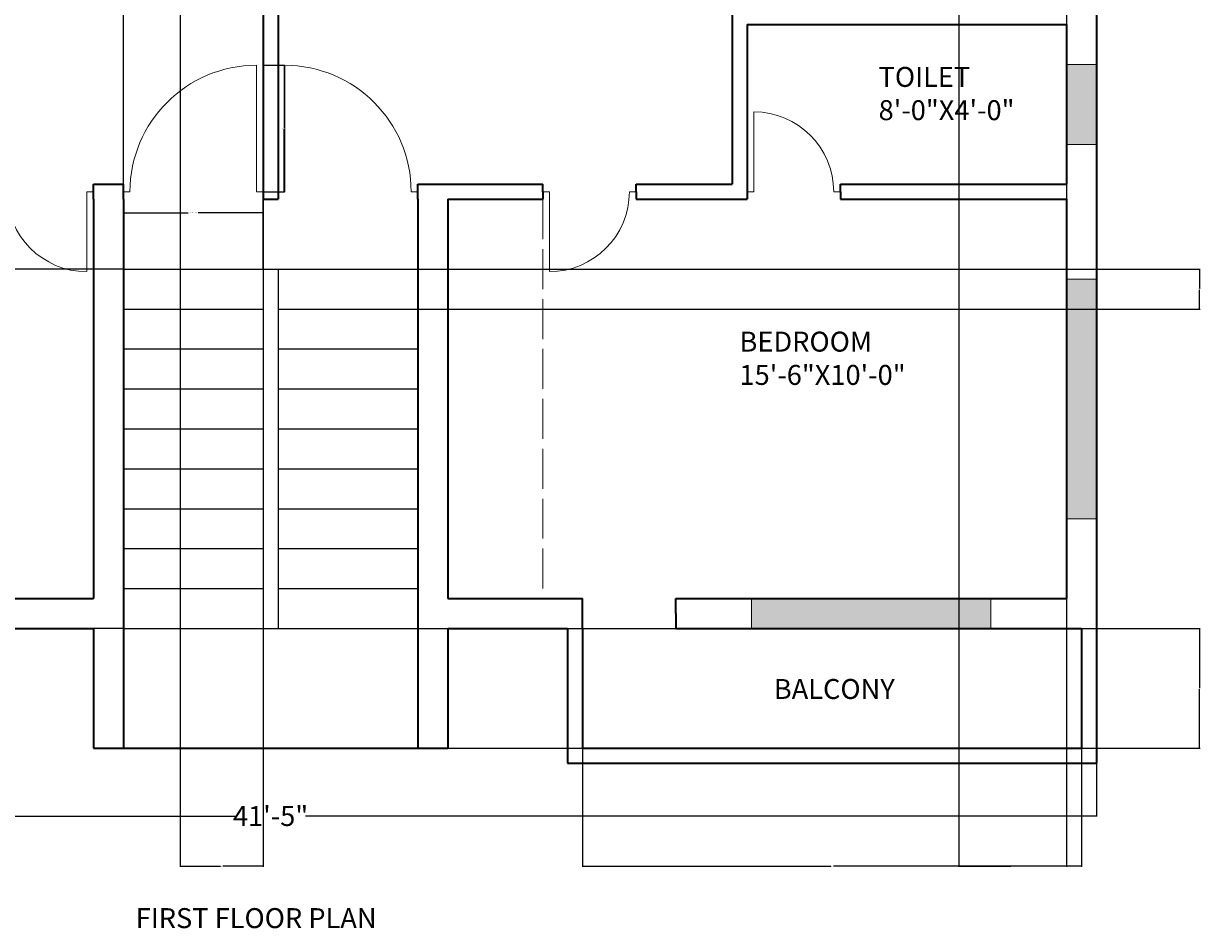
# Model space of a CAD drawing. Units: inches. Extents: x -89 to 565, y -517 to 71.
# Tile 2 of 3: x 211 to 565, y -517 to -245. Entities that reach past the tile are written whole.
import ezdxf

# ---------------------------------------------------------------- set-up
doc = ezdxf.new("R2010")
doc.units = ezdxf.units.IN
doc.header["$MEASUREMENT"] = 0
doc.linetypes.add('ACAD_ISO02W100', pattern=[15, 12, -3])
for name, color, linetype, lineweight in [('A-ANNO-DIMS', 2, 'Continuous', 18), ('A-ANNO-TEXT', 7, 'Continuous', 25), ('A-AREA-IDEN', 7, 'Continuous', 18), ('A-DOOR', 4, 'Continuous', 18), ('A-FLOR-OVHD', 8, 'ACAD_ISO02W100', 18), ('A-FLOR-STRS', 7, 'Continuous', 25), ('A-GLAZ', 3, 'Continuous', 18), ('A-GLAZ-PATT', 9, 'Continuous', 13), ('A-WALL', 7, 'Continuous', 35)]:
    doc.layers.add(name, color=color, linetype=linetype, lineweight=lineweight)
doc.styles.get("Standard").update_dxf_attribs({"font": 'arial.ttf'})
doc.dimstyles.get("Standard").update_dxf_attribs({"dimtxt": 0.18, "dimasz": 0.18, "dimexe": 0.18, "dimexo": 0.0625, "dimgap": 0.09, "dimtad": 0, "dimtih": 1, "dimtoh": 1, "dimdec": 0, "dimzin": 0, "dimdsep": 46, "dimlunit": 3, "dimtxsty": 'Standard', "dimcen": 0.09, "dimadec": 0, "dimazin": 0, "dimtfac": 1, "dimtdec": 0, "dimtofl": 0, "dimtmove": 0, "dimatfit": 3, "dimfxl": 1, "dimtolj": 1, "dimtzin": 0, "dimarcsym": 0})

# ---------------------------------------------------------------- blocks, each defined once
blk = doc.blocks.new('*D2')
at = {"layer": 'A-ANNO-DIMS', "color": 0, "lineweight": -2, "transparency": 16777216}
for p, q in [((37.09, -467.65), (37.09, -483.62)), ((533.59, -467.65), (533.59, -483.62)), ((37.27, -483.44), (274.83, -483.44)), ((533.41, -483.44), (295.86, -483.44))]:
    blk.add_line(p, q, dxfattribs=at)
at = {"layer": 'A-ANNO-DIMS', "color": 0, "transparency": 16777216}
for points in [[(37.27, -483.41), (37.27, -483.47), (37.09, -483.44)], [(533.41, -483.41), (533.41, -483.47), (533.59, -483.44)]]:
    blk.add_solid(points, dxfattribs=at)
at = {"layer": 'Defpoints', "color": 0, "transparency": 16777216}
for p in [(37.09, -467.59), (533.59, -467.59), (533.59, -483.44)]:
    blk.add_point(p, dxfattribs=at)
at = {"layer": 'A-ANNO-DIMS', "color": 0, "transparency": 16777216, "insert": (285.34, -483.44), "char_height": 6, "attachment_point": 5}
blk.add_mtext('\\A1;41\'-5"', dxfattribs=at)
blk = doc.blocks.new('DOOR-SWING-24IN')
for p, q in [((0, 0), (0, 24)), ((-24, 0), (-26, 0)), ((2, 0), (0, 0))]:
    blk.add_line(p, q)
blk.add_arc((0, 0), 24, 90, 180)
blk = doc.blocks.new('DOOR-ENTRY-38IN')
for p, q in [((0, 0), (0, 38)), ((-40, 0), (-38, 0)), ((2, 0), (0, 0))]:
    blk.add_line(p, q)
blk.add_arc((0, 0), 38, 90, 180)
blk = doc.blocks.new('*D12')
at = {"layer": 'A-ANNO-DIMS', "color": 0, "lineweight": -2, "transparency": 16777216}
for p, q in [((241.09, -295.9), (241.09, -302.32)), ((283.09, -295.9), (283.09, -302.32)), ((241.27, -302.14), (260.59, -302.14)), ((282.91, -302.14), (263.6, -302.14))]:
    blk.add_line(p, q, dxfattribs=at)
at = {"layer": 'A-ANNO-DIMS', "color": 0, "transparency": 16777216}
for points in [[(241.27, -302.11), (241.27, -302.17), (241.09, -302.14)], [(282.91, -302.11), (282.91, -302.17), (283.09, -302.14)]]:
    blk.add_solid(points, dxfattribs=at)
at = {"layer": 'Defpoints', "color": 0, "transparency": 16777216}
for p in [(241.09, -295.84), (283.09, -295.84), (283.09, -302.14)]:
    blk.add_point(p, dxfattribs=at)
at = {"layer": 'A-ANNO-DIMS', "color": 0, "transparency": 16777216, "insert": (262.09, -302.14), "char_height": 0.18, "attachment_point": 5}
blk.add_mtext('\\A1;ENTRY DOOR 3\'-6" TYP.', dxfattribs=at)
blk = doc.blocks.new('*D13')
at = {"layer": 'A-ANNO-DIMS', "color": 0, "lineweight": -2, "transparency": 16777216}
for p, q in [((283.16, -257.84), (289.57, -257.84)), ((289.39, -258.02), (289.39, -276.65)), ((289.39, -295.66), (289.39, -277.02)), ((283.16, -295.84), (289.57, -295.84))]:
    blk.add_line(p, q, dxfattribs=at)
at = {"layer": 'A-ANNO-DIMS', "color": 0, "transparency": 16777216}
for points in [[(289.36, -258.02), (289.42, -258.02), (289.39, -257.84)], [(289.36, -295.66), (289.42, -295.66), (289.39, -295.84)]]:
    blk.add_solid(points, dxfattribs=at)
at = {"layer": 'Defpoints', "color": 0, "transparency": 16777216}
for p in [(283.09, -257.84), (289.39, -257.84), (283.09, -295.84)]:
    blk.add_point(p, dxfattribs=at)
at = {"layer": 'A-ANNO-DIMS', "color": 0, "transparency": 16777216, "insert": (289.39, -276.84), "char_height": 0.18, "attachment_point": 5}
blk.add_mtext('\\A1;3\'-2" TYP.', dxfattribs=at)
blk = doc.blocks.new('*D26')
at = {"layer": 'A-ANNO-DIMS', "color": 0, "lineweight": -2, "transparency": 16777216}
for p, q in [((241.09, -319.02), (241.09, 70.54)), ((241.27, 70.36), (261.76, 70.36)), ((282.91, 70.36), (262.42, 70.36)), ((283.09, -319.02), (283.09, 70.54))]:
    blk.add_line(p, q, dxfattribs=at)
at = {"layer": 'A-ANNO-DIMS', "color": 0, "transparency": 16777216}
for points in [[(241.27, 70.39), (241.27, 70.33), (241.09, 70.36)], [(282.91, 70.39), (282.91, 70.33), (283.09, 70.36)]]:
    blk.add_solid(points, dxfattribs=at)
at = {"layer": 'Defpoints', "color": 0, "transparency": 16777216}
for p in [(283.09, 70.36), (241.09, -319.09), (283.09, -319.09)]:
    blk.add_point(p, dxfattribs=at)
at = {"layer": 'A-ANNO-DIMS', "color": 0, "transparency": 16777216, "insert": (262.09, 70.36), "char_height": 0.18, "attachment_point": 5}
blk.add_mtext('\\A1;3\'-6"', dxfattribs=at)
blk = doc.blocks.new('*D27')
at = {"layer": 'A-ANNO-DIMS', "color": 0, "lineweight": -2, "transparency": 16777216}
for p, q in [((241.03, -319.09), (-27.04, -319.09)), ((-26.86, -319.27), (-26.86, -372.9)), ((-26.86, -426.91), (-26.86, -373.27)), ((241.03, -427.09), (-27.04, -427.09))]:
    blk.add_line(p, q, dxfattribs=at)
at = {"layer": 'A-ANNO-DIMS', "color": 0, "transparency": 16777216}
for points in [[(-26.89, -319.27), (-26.83, -319.27), (-26.86, -319.09)], [(-26.89, -426.91), (-26.83, -426.91), (-26.86, -427.09)]]:
    blk.add_solid(points, dxfattribs=at)
at = {"layer": 'Defpoints', "color": 0, "transparency": 16777216}
for p in [(241.09, -319.09), (-26.86, -427.09), (241.09, -427.09)]:
    blk.add_point(p, dxfattribs=at)
at = {"layer": 'A-ANNO-DIMS', "color": 0, "transparency": 16777216, "insert": (-26.86, -373.09), "char_height": 0.18, "attachment_point": 5}
blk.add_mtext('\\A1;9\'-0"', dxfattribs=at)
blk = doc.blocks.new('*D28')
at = {"layer": 'A-ANNO-DIMS', "color": 0, "lineweight": -2, "transparency": 16777216}
for p, q in [((329.66, -427.09), (564.72, -427.09)), ((564.54, -427.27), (564.54, -444.9)), ((564.54, -462.91), (564.54, -445.27)), ((329.66, -463.09), (564.72, -463.09))]:
    blk.add_line(p, q, dxfattribs=at)
at = {"layer": 'A-ANNO-DIMS', "color": 0, "transparency": 16777216}
for points in [[(564.51, -427.27), (564.57, -427.27), (564.54, -427.09)], [(564.51, -462.91), (564.57, -462.91), (564.54, -463.09)]]:
    blk.add_solid(points, dxfattribs=at)
at = {"layer": 'Defpoints', "color": 0, "transparency": 16777216}
for p in [(329.59, -427.09), (564.54, -427.09), (329.59, -463.09)]:
    blk.add_point(p, dxfattribs=at)
at = {"layer": 'A-ANNO-DIMS', "color": 0, "transparency": 16777216, "insert": (564.54, -445.09), "char_height": 0.18, "attachment_point": 5}
blk.add_mtext('\\A1;3\'-0"', dxfattribs=at)
blk = doc.blocks.new('*D29')
at = {"layer": 'A-ANNO-DIMS', "color": 0, "lineweight": -2, "transparency": 16777216}
for p, q in [((329.66, -319.09), (564.72, -319.09)), ((564.54, -319.27), (564.54, -324.9)), ((564.54, -330.91), (564.54, -325.27)), ((329.66, -331.09), (564.72, -331.09))]:
    blk.add_line(p, q, dxfattribs=at)
at = {"layer": 'A-ANNO-DIMS', "color": 0, "transparency": 16777216}
for points in [[(564.51, -319.27), (564.57, -319.27), (564.54, -319.09)], [(564.51, -330.91), (564.57, -330.91), (564.54, -331.09)]]:
    blk.add_solid(points, dxfattribs=at)
at = {"layer": 'Defpoints', "color": 0, "transparency": 16777216}
for p in [(329.59, -319.09), (329.59, -331.09), (564.54, -331.09)]:
    blk.add_point(p, dxfattribs=at)
at = {"layer": 'A-ANNO-DIMS', "color": 0, "transparency": 16777216, "insert": (564.54, -325.09), "char_height": 0.18, "attachment_point": 5}
blk.add_mtext('\\A1;1\'-0"', dxfattribs=at)
blk = doc.blocks.new('*D31')
at = {"layer": 'A-ANNO-DIMS', "color": 0, "lineweight": -2, "transparency": 16777216}
for p, q in [((379.09, -463.15), (379.09, -498.72)), ((529.09, -463.15), (529.09, -498.72)), ((379.27, -498.54), (453.7, -498.54)), ((528.91, -498.54), (454.48, -498.54))]:
    blk.add_line(p, q, dxfattribs=at)
at = {"layer": 'A-ANNO-DIMS', "color": 0, "transparency": 16777216}
for points in [[(379.27, -498.51), (379.27, -498.57), (379.09, -498.54)], [(528.91, -498.51), (528.91, -498.57), (529.09, -498.54)]]:
    blk.add_solid(points, dxfattribs=at)
at = {"layer": 'Defpoints', "color": 0, "transparency": 16777216}
for p in [(379.09, -463.09), (529.09, -463.09), (529.09, -498.54)]:
    blk.add_point(p, dxfattribs=at)
at = {"layer": 'A-ANNO-DIMS', "color": 0, "transparency": 16777216, "insert": (454.09, -498.54), "char_height": 0.18, "attachment_point": 5}
blk.add_mtext('\\A1;12\'-6"', dxfattribs=at)
blk = doc.blocks.new('*D32')
at = {"layer": 'A-ANNO-DIMS', "color": 0, "lineweight": -2, "transparency": 16777216}
for p, q in [((529.16, -427.09), (564.72, -427.09)), ((564.54, -427.27), (564.54, -444.9)), ((564.54, -462.91), (564.54, -445.27)), ((529.16, -463.09), (564.72, -463.09))]:
    blk.add_line(p, q, dxfattribs=at)
at = {"layer": 'A-ANNO-DIMS', "color": 0, "transparency": 16777216}
for points in [[(564.51, -427.27), (564.57, -427.27), (564.54, -427.09)], [(564.51, -462.91), (564.57, -462.91), (564.54, -463.09)]]:
    blk.add_solid(points, dxfattribs=at)
at = {"layer": 'Defpoints', "color": 0, "transparency": 16777216}
for p in [(529.09, -427.09), (564.54, -427.09), (529.09, -463.09)]:
    blk.add_point(p, dxfattribs=at)
at = {"layer": 'A-ANNO-DIMS', "color": 0, "transparency": 16777216, "insert": (564.54, -445.09), "char_height": 0.18, "attachment_point": 5}
blk.add_mtext('\\A1;3\'-0"', dxfattribs=at)
blk = doc.blocks.new('*D34')
at = {"layer": 'A-ANNO-DIMS', "color": 0, "lineweight": -2, "transparency": 16777216}
for p, q in [((258.18, -94.15), (258.18, -498.72)), ((283.09, -94.15), (283.09, -498.72)), ((258.36, -498.54), (270.31, -498.54)), ((282.91, -498.54), (270.97, -498.54))]:
    blk.add_line(p, q, dxfattribs=at)
at = {"layer": 'A-ANNO-DIMS', "color": 0, "transparency": 16777216}
for points in [[(258.36, -498.51), (258.36, -498.57), (258.18, -498.54)], [(282.91, -498.51), (282.91, -498.57), (283.09, -498.54)]]:
    blk.add_solid(points, dxfattribs=at)
at = {"layer": 'Defpoints', "color": 0, "transparency": 16777216}
for p in [(258.18, -94.09), (283.09, -94.09), (283.09, -498.54)]:
    blk.add_point(p, dxfattribs=at)
at = {"layer": 'A-ANNO-DIMS', "color": 0, "transparency": 16777216, "insert": (270.64, -498.54), "char_height": 0.18, "attachment_point": 5}
blk.add_mtext('\\A1;2\'-1"', dxfattribs=at)
blk = doc.blocks.new('*D35')
at = {"layer": 'A-ANNO-DIMS', "color": 0, "lineweight": -2, "transparency": 16777216}
for p, q in [((492.2, -127.15), (492.2, -498.72)), ((524.59, -127.15), (524.59, -498.72)), ((492.38, -498.54), (507.86, -498.54)), ((524.41, -498.54), (508.94, -498.54))]:
    blk.add_line(p, q, dxfattribs=at)
at = {"layer": 'A-ANNO-DIMS', "color": 0, "transparency": 16777216}
for points in [[(492.38, -498.51), (492.38, -498.57), (492.2, -498.54)], [(524.41, -498.51), (524.41, -498.57), (524.59, -498.54)]]:
    blk.add_solid(points, dxfattribs=at)
at = {"layer": 'Defpoints', "color": 0, "transparency": 16777216}
for p in [(492.2, -127.09), (524.59, -127.09), (524.59, -498.54)]:
    blk.add_point(p, dxfattribs=at)
at = {"layer": 'A-ANNO-DIMS', "color": 0, "transparency": 16777216, "insert": (508.4, -498.54), "char_height": 0.18, "attachment_point": 5}
blk.add_mtext('\\A1;2\'-8 1/2"', dxfattribs=at)

msp = doc.modelspace()

# ---------------------------------------------------------------- hatches: boundary and pattern name
at = {"layer": 'A-GLAZ-PATT'}
h = msp.add_hatch(dxfattribs=at)
h.set_pattern_fill('GOST_WOOD', color=256)
h.set_pattern_definition([(90, (0, 0), (6, -4e-16), [10, -2]), (90, (2, -2), (6, -4e-16), [6, -1.5, 3, -1.5]), (90, (4, -5), (6, -4e-16), [10, -2])])
h.paths.add_polyline_path([(46.09, -73.09), (41.59, -73.09), (37.09, -73.09), (37.09, -133.09), (41.59, -133.09), (46.09, -133.09)])
h.paths.add_polyline_path([(46.09, -175.84), (41.59, -175.84), (37.09, -175.84), (37.09, -223.84), (41.59, -223.84), (46.09, -223.84)])
h.paths.add_polyline_path([(46.09, -257.59), (41.59, -257.59), (37.09, -257.59), (37.09, -281.59), (41.59, -281.59), (46.09, -281.59)])
h.paths.add_polyline_path([(140.84, -418.09), (68.84, -418.09), (68.84, -422.59), (68.84, -427.09), (140.84, -427.09), (140.84, -422.59)])
h.paths.add_polyline_path([(501.84, -418.09), (429.84, -418.09), (429.84, -422.59), (429.84, -427.09), (501.84, -427.09), (501.84, -422.59)])
h.paths.add_polyline_path([(533.59, -322.09), (529.09, -322.09), (524.59, -322.09), (524.59, -394.09), (529.09, -394.09), (533.59, -394.09)])
h.paths.add_polyline_path([(533.59, -257.59), (529.09, -257.59), (524.59, -257.59), (524.59, -281.59), (529.09, -281.59), (533.59, -281.59)])
h.paths.add_polyline_path([(533.59, -205.09), (529.09, -205.09), (524.59, -205.09), (524.59, -229.09), (529.09, -229.09), (533.59, -229.09)])
h.paths.add_polyline_path([(533.59, -148.09), (529.09, -148.09), (524.59, -148.09), (524.59, -172.09), (529.09, -172.09), (533.59, -172.09)])
h.paths.add_polyline_path([(533.59, -26.59), (529.09, -26.59), (524.59, -26.59), (524.59, -98.59), (529.09, -98.59), (533.59, -98.59)])
h.paths.add_polyline_path([(421.09, 10.91), (365.78, 10.91), (365.78, 1.91), (421.09, 1.91)])
h.paths.add_polyline_path([(194.59, 10.91), (170.59, 10.91), (170.59, 1.91), (194.59, 1.91)])

# ---------------------------------------------------------------- linework, layer by layer
at = {"layer": 'A-FLOR-OVHD'}
msp.add_line((367.17, -298.09), (367.17, -418.09), dxfattribs=at)
at = {"layer": 'A-FLOR-STRS'}
for p, q in [((241.09, -319.09), (329.59, -319.09)), ((283.09, -319.09), (283.09, -427.09)), ((287.59, -319.09), (287.59, -427.09)), ((241.09, -331.09), (283.09, -331.09)), ((287.59, -331.09), (329.59, -331.09)), ((241.09, -343.09), (283.09, -343.09)), ((287.59, -343.09), (329.59, -343.09)), ((241.09, -355.09), (283.09, -355.09)), ((287.59, -355.09), (329.59, -355.09)), ((241.09, -367.09), (283.09, -367.09)), ((287.59, -367.09), (329.59, -367.09)), ((241.09, -379.09), (283.09, -379.09)), ((287.59, -379.09), (329.59, -379.09)), ((241.09, -391.09), (283.09, -391.09)), ((287.59, -391.09), (329.59, -391.09)), ((241.09, -403.09), (283.09, -403.09)), ((287.59, -403.09), (329.59, -403.09)), ((241.09, -415.09), (283.09, -415.09)), ((287.59, -415.09), (329.59, -415.09)), ((241.09, -427.09), (329.59, -427.09))]:
    msp.add_line(p, q, dxfattribs=at)
at = {"layer": 'A-GLAZ'}
for p, q in [((529.09, -257.59), (524.59, -257.59)), ((529.09, -257.59), (533.59, -257.59)), ((529.09, -281.59), (524.59, -281.59)), ((529.09, -281.59), (533.59, -281.59)), ((529.09, -322.09), (524.59, -322.09)), ((529.09, -322.09), (533.59, -322.09)), ((529.09, -394.09), (524.59, -394.09)), ((529.09, -394.09), (533.59, -394.09)), ((429.84, -422.59), (429.84, -418.09)), ((501.84, -422.59), (501.84, -418.09)), ((429.84, -422.59), (429.84, -427.09)), ((501.84, -422.59), (501.84, -427.09))]:
    msp.add_line(p, q, dxfattribs=at)
at = {"layer": 'A-WALL'}
for p, q in [((533.59, 10.91), (533.59, -467.59)), ((283.09, -98.59), (283.09, -298.09)), ((287.59, -131.59), (287.59, -298.09)), ((424.09, -188.59), (424.09, -293.59)), ((428.59, -245.59), (524.59, -245.59)), ((428.59, -245.59), (428.59, -298.09)), ((524.59, -245.59), (524.59, -293.59)), ((232.09, -298.09), (232.09, -293.59)), ((232.09, -293.59), (241.09, -293.59)), ((241.09, -298.09), (241.09, -293.59)), ((329.59, -298.09), (329.59, -293.59)), ((329.59, -293.59), (367.17, -293.59)), ((367.17, -295.84), (367.17, -293.59)), ((395.17, -295.84), (395.17, -293.59)), ((395.17, -293.59), (424.09, -293.59)), ((456.59, -295.84), (456.59, -293.59)), ((456.59, -293.59), (524.59, -293.59)), ((367.17, -295.84), (367.17, -298.09)), ((395.17, -295.84), (395.17, -298.09)), ((456.59, -295.84), (456.59, -298.09)), ((232.09, -298.09), (232.09, -418.09)), ((241.09, -298.09), (241.09, -463.09)), ((283.09, -298.09), (287.59, -298.09)), ((329.59, -298.09), (329.59, -463.09)), ((338.59, -298.09), (338.59, -418.09)), ((338.59, -298.09), (367.17, -298.09)), ((395.17, -298.09), (428.59, -298.09)), ((456.59, -298.09), (524.59, -298.09)), ((524.59, -298.09), (524.59, -418.09)), ((191.59, -418.09), (232.09, -418.09)), ((338.59, -418.09), (379.09, -418.09)), ((379.09, -427.09), (379.09, -418.09)), ((407.09, -422.59), (407.09, -418.09)), ((407.09, -418.09), (524.59, -418.09)), ((407.09, -422.59), (407.09, -427.09)), ((196.09, -427.09), (232.09, -427.09)), ((232.09, -427.09), (232.09, -463.09)), ((338.59, -427.09), (374.59, -427.09)), ((338.59, -427.09), (338.59, -463.09)), ((374.59, -427.09), (374.59, -467.59)), ((379.09, -427.09), (379.09, -463.09)), ((407.09, -427.09), (529.09, -427.09)), ((529.09, -427.09), (529.09, -463.09)), ((232.09, -463.09), (338.59, -463.09)), ((379.09, -463.09), (529.09, -463.09)), ((374.59, -467.59), (533.59, -467.59))]:
    msp.add_line(p, q, dxfattribs=at)

# ---------------------------------------------------------------- block references
at = {"layer": 'A-DOOR'}
msp.add_blockref('DOOR-ENTRY-38IN', (281.09, -295.84), dxfattribs=at)
at = {"layer": 'A-DOOR', "extrusion": (0, 0, -1), "zscale": -1}
for name, p in [('DOOR-ENTRY-38IN', (-289.59, -295.84)), ('DOOR-SWING-24IN', (-430.59, -295.84))]:
    msp.add_blockref(name, p, dxfattribs=at)
at = {"layer": 'A-DOOR', "extrusion": (0, 0, -1), "zscale": -1, "rotation": 180}
msp.add_blockref('DOOR-SWING-24IN', (-230.09, -295.84), dxfattribs=at)
at = {"layer": 'A-DOOR', "rotation": 180}
msp.add_blockref('DOOR-SWING-24IN', (369.17, -295.84), dxfattribs=at)

# ---------------------------------------------------------------- texts
at = {"layer": 'A-ANNO-TEXT', "insert": (244.81, -511.13), "char_height": 6, "attachment_point": 1}
msp.add_mtext('FIRST FLOOR PLAN', dxfattribs=at)
at = {"layer": 'A-AREA-IDEN', "char_height": 6, "attachment_point": 1}
for s, insert in [('TOILET\\P8\'-0"X4\'-0"', (468.08, -258.32)), ('BEDROOM\\P15\'-6"X10\'-0"', (426.27, -337.88)), ('BALCONY', (436.58, -442.27))]:
    msp.add_mtext(s, dxfattribs=dict(at, insert=insert))

# ---------------------------------------------------------------- dimensions: what is measured, and where the dimension line sits
at = {"layer": 'A-ANNO-DIMS'}
for base, p1, p2, override, picture, middle in [((283.09, 70.36), (241.09, -319.09), (283.09, -319.09), {"dimdec": 1, "dimlfac": 1, "dimrnd": 0, "dimzin": 1, "dimdsep": 46, "dimlunit": 4, "dimfrac": 2}, '*D26', (262.09, 70.36)), ((283.09, -498.54), (258.18, -94.09), (283.09, -94.09), {"dimdec": 1, "dimlfac": 1, "dimrnd": 0, "dimzin": 1, "dimdsep": 46, "dimlunit": 4, "dimfrac": 2}, '*D34', (270.64, -498.54)), ((524.59, -498.54), (492.2, -127.09), (524.59, -127.09), {"dimdec": 1, "dimlfac": 1, "dimrnd": 0, "dimzin": 1, "dimdsep": 46, "dimlunit": 4, "dimfrac": 2}, '*D35', (508.4, -498.54)), ((529.09, -498.54), (379.09, -463.09), (529.09, -463.09), {"dimdec": 1, "dimlfac": 1, "dimrnd": 0, "dimzin": 1, "dimdsep": 46, "dimlunit": 4, "dimfrac": 2}, '*D31', (454.09, -498.54)), ((533.59381792, -483.44106033), (37.09381792, -467.58551125), (533.59381792, -467.58551125), {"dimtxt": 6, "dimclrd": 0, "dimclre": 0, "dimclrt": 0}, '*D2', (285.34381792, -483.44106033))]:
    dim = msp.add_linear_dim(base=base, p1=p1, p2=p2, dimstyle='Standard', override=override, dxfattribs=at)
    dim.commit()
    dim.dimension.update_dxf_attribs({"geometry": picture, "text_midpoint": middle})
dim = msp.add_linear_dim(base=(289.39, -257.84), p1=(283.09, -295.84), p2=(283.09, -257.84), angle=90, text='<> TYP.', dimstyle='Standard', override={"dimdec": 1, "dimlfac": 1, "dimrnd": 0, "dimzin": 1, "dimdsep": 46, "dimlunit": 4, "dimfrac": 2}, dxfattribs=at)
dim.commit()
dim.dimension.update_dxf_attribs({"geometry": '*D13', "text_midpoint": (289.39, -276.84)})
dim = msp.add_linear_dim(base=(283.09, -302.14), p1=(241.09, -295.84), p2=(283.09, -295.84), text='ENTRY DOOR <> TYP.', dimstyle='Standard', override={"dimdec": 1, "dimlfac": 1, "dimrnd": 0, "dimzin": 1, "dimdsep": 46, "dimlunit": 4, "dimfrac": 2}, dxfattribs=at)
dim.commit()
dim.dimension.update_dxf_attribs({"geometry": '*D12', "text_midpoint": (262.09, -302.14)})
for base, p1, p2, picture, middle in [((-26.86, -427.09), (241.09, -319.09), (241.09, -427.09), '*D27', (-26.86, -373.09)), ((564.54, -331.09), (329.59, -319.09), (329.59, -331.09), '*D29', (564.54, -325.09)), ((564.54, -427.09), (329.59, -463.09), (329.59, -427.09), '*D28', (564.54, -445.09)), ((564.54, -427.09), (529.09, -463.09), (529.09, -427.09), '*D32', (564.54, -445.09))]:
    dim = msp.add_linear_dim(base=base, p1=p1, p2=p2, angle=90, dimstyle='Standard', override={"dimdec": 1, "dimlfac": 1, "dimrnd": 0, "dimzin": 1, "dimdsep": 46, "dimlunit": 4, "dimfrac": 2}, dxfattribs=at)
    dim.commit()
    dim.dimension.update_dxf_attribs({"geometry": picture, "text_midpoint": middle})

doc.saveas('drawing.dxf')
